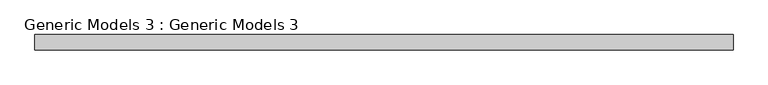
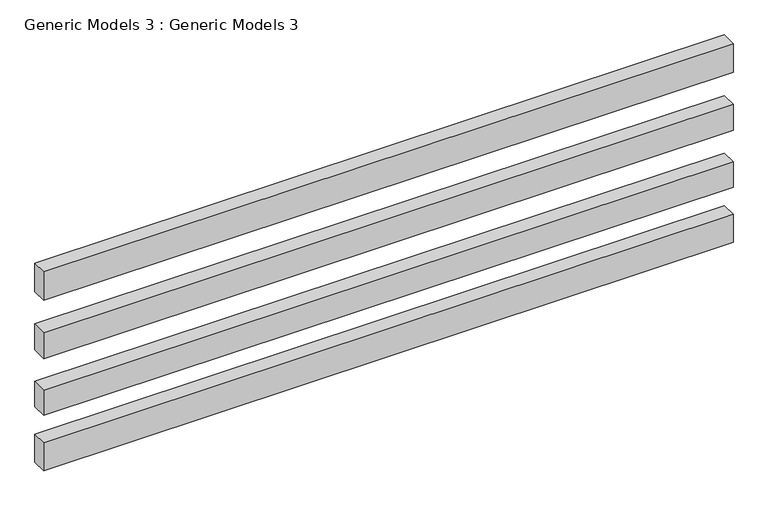
"""IFC4 building model written with IfcOpenShell, lengths in millimetres: proxy geometry, Generic Models 3 : Generic Models 3."""

from ifc_helpers import new_model, si_unit, frame, origin, place, context, project, spatial, polyline, outline, extrude, source, transform, mapped, element, save


def generic_models_3_generic_models_3_88f68afe(model_context):
    return source(origin(), model_context, "Body", "SweptSolid", [
        extrude(outline(polyline([(-10339.149223, -14905.0922199), (-10339.149223, -14981.2922199), (-13816.7150098, -14981.2922199), (-13816.7150098, -14905.0922199), (-10339.149223, -14905.0922199)])), frame((0.0, 0.0, 7295.1995979), z_axis=(0.0, 0.0, 1.0), x_axis=(1.0, 0.0, 0.0)), (0.0, 0.0, 1.0), 152.4),
        extrude(outline(polyline([(-10339.149223, -14905.0922199), (-10339.149223, -14981.2922199), (-13816.7150098, -14981.2922199), (-13816.7150098, -14905.0922199), (-10339.149223, -14905.0922199)])), frame((0.0, 0.0, 6985.5530079), z_axis=(0.0, 0.0, 1.0), x_axis=(1.0, 0.0, 0.0)), (0.0, 0.0, 1.0), 138.2491276),
        extrude(outline(polyline([(-10339.149223, -14905.0922199), (-10339.149223, -14981.2922199), (-13816.7150098, -14981.2922199), (-13816.7150098, -14905.0922199), (-10339.149223, -14905.0922199)])), frame((0.0, 0.0, 6682.3821213), z_axis=(0.0, 0.0, 1.0), x_axis=(1.0, 0.0, 0.0)), (0.0, 0.0, 1.0), 134.6929761),
        extrude(outline(polyline([(-10339.149223, -14905.0922199), (-10339.149223, -14981.2922199), (-13816.7150098, -14981.2922199), (-13816.7150098, -14905.0922199), (-10339.149223, -14905.0922199)])), frame((0.0, 0.0, 6387.5684897), z_axis=(0.0, 0.0, 1.0), x_axis=(1.0, 0.0, 0.0)), (0.0, 0.0, 1.0), 149.2734963),
    ])


if __name__ == "__main__":
    model = new_model("IFC4")
    model_context = context("Model", 3, world=origin())
    ifc_project = project(units=[si_unit("LENGTHUNIT", "METRE", prefix="MILLI")], contexts=[model_context])
    site = spatial("IfcSite", under=ifc_project)
    building = spatial("IfcBuilding", under=site)
    placement = place(None, origin())
    generic_models_3_generic_models_3_shape = generic_models_3_generic_models_3_88f68afe(model_context)
    element("IfcBuildingElementProxy", 1, Name="Generic Models 3 : Generic Models 3", ObjectType="Generic Models 3 : Generic Models 3", at=placement, inside=building, context=model_context, shape_type="MappedRepresentation", body=[
        mapped(generic_models_3_generic_models_3_shape, transform((0.0, 0.0, 0.0), x_axis=(1.0, 0.0, 0.0), y_axis=(0.0, 1.0, 0.0), z_axis=(0.0, 0.0, 1.0))),
    ])
    save(model, "model.ifc")
